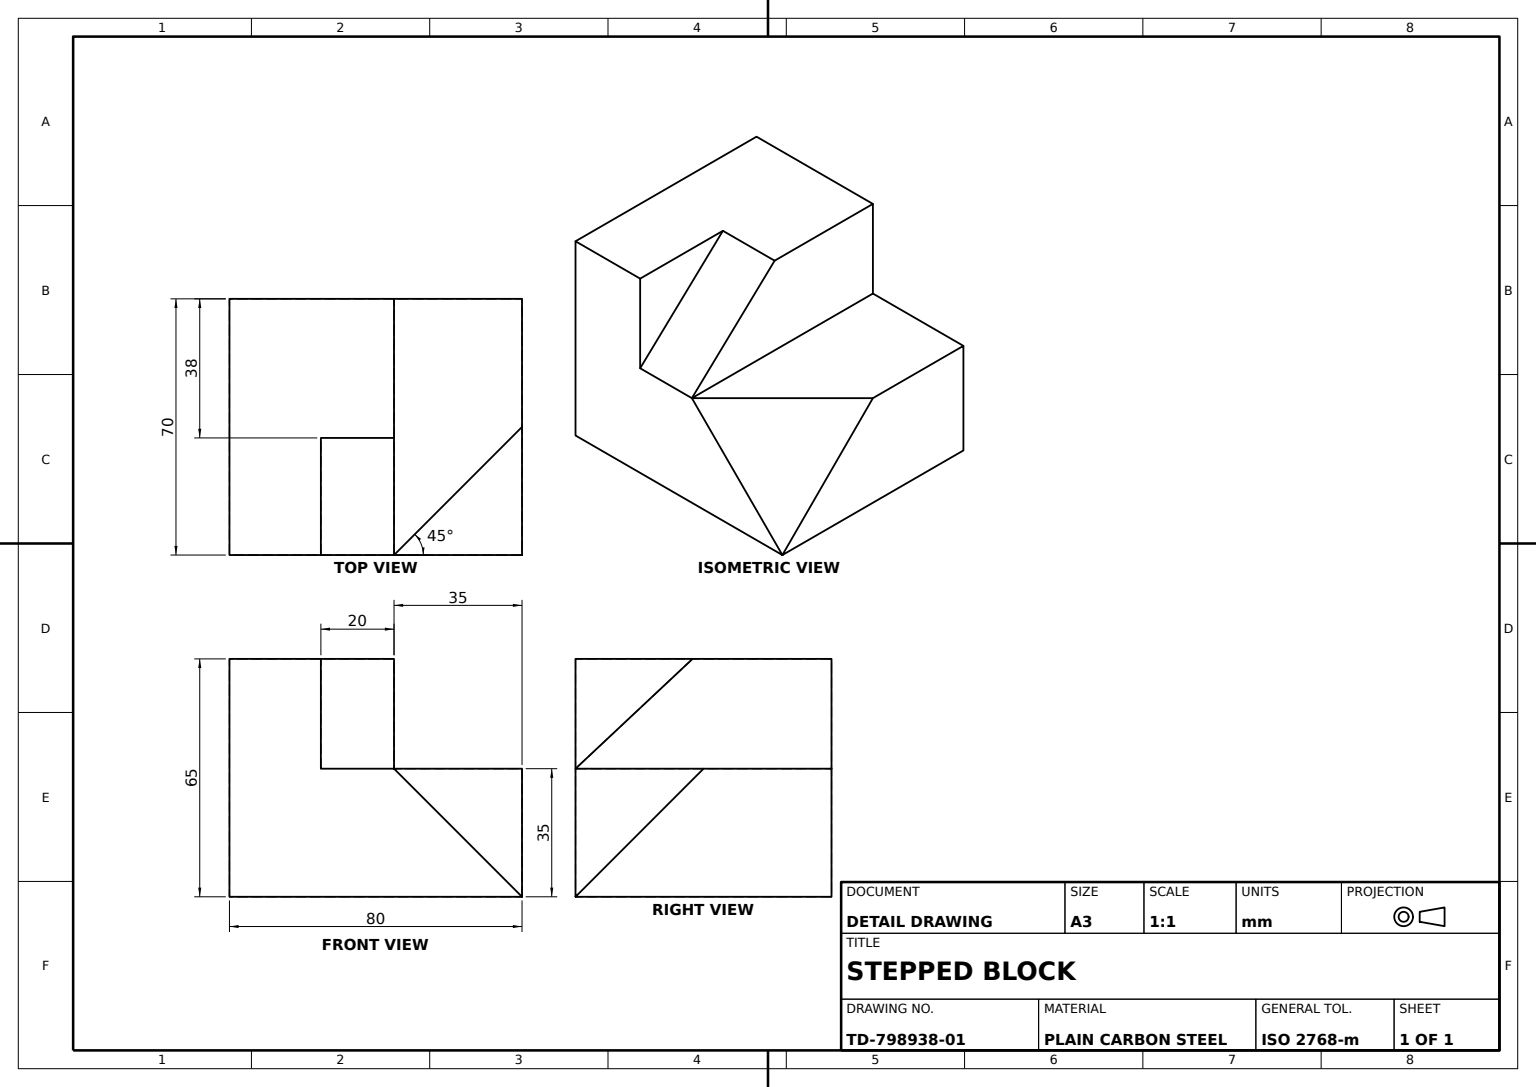
SolidWorks part; units mm, degrees
material "Plain Carbon Steel"
ref_plane "Front Plane" through (0, 0, 0) normal (0, 0, 1) x (1, 0, 0)
ref_plane "Top Plane" through (0, 0, 0) normal (0, 1, 0) x (1, 0, 0)
ref_plane "Right Plane" through (0, 0, 0) normal (1, 0, 0) x (0, 0, -1)
sketch "Block Profile Sketch 70x65" plane through (0, 0, 0) normal (0, 0, 1) x (1, 0, 0)
  line L0 (0, 0) -> (70, 0)
  line L1 (70, 0) -> (70, 65)
  line L2 (70, 65) -> (0, 65)
  line L3 (0, 65) -> (0, 0)
  dimension "D1" = 65
  dimension "D2" = 70
extrude "Base Block 70x65x80" add sketch "Block Profile Sketch 70x65" along normal mid plane 80
sketch "Upper Step Sketch" plane through (0, 0, 40) normal (0, 0, 1) x (1, 0, 0)
  line L0 (0, 35) -> (70, 35)
  line L1 (0, 65) -> (0, 0) construction
  line L2 (70, 0) -> (70, 65) construction
  line L3 (70, 35) -> (70, 65)
  line L4 (70, 65) -> (0, 65)
  line L5 (0, 65) -> (0, 35)
  line L6 (0, 0) -> (70, 0) construction
  dimension "D1" = 35
extrude "Upper Step Cut 35" cut sketch "Upper Step Sketch" against normal blind 35
sketch "Lower Step Sketch" plane through (0, 0, 5) normal (0, 0, 1) x (1, 0, 0)
  line L0 (0, 35) -> (32, 65)
  line L1 (70, 65) -> (0, 65) construction
  line L2 (70, 35) -> (70, 65) construction
  line L6 (0, 65) -> (0, 35) construction
  line L7 (32, 65) -> (0, 65)
  line L8 (0, 65) -> (0, 35)
  dimension "D1" = 38
extrude "Lower Step Cut 20" cut sketch "Lower Step Sketch" against normal blind 20
sketch3d "Corner Cut Reference 3D Sketch"
  line L0 (0, 0, 40) -> (35, 35, 40) construction
  line L1 (0, 35, 40) -> (70, 35, 40) construction
  line L2 (35, 35, 40) -> (0, 35, 5) construction
  line L3 (0, 35, 5) -> (0, 0, 40) construction
  line L4 (70, 35, 5) -> (70, 35, 40) construction
  dimension "D1" = 35
ref_plane "Corner Cut Plane" through (-13.3333, 13.3333, 13.3333) normal (0.5774, -0.5774, -0.5774) x (-0.8165, -0.4082, -0.4082)
sketch "Corner Cut Sketch" plane through (-13.3333, 13.3333, 13.3333) normal (0.5774, -0.5774, -0.5774) x (-0.8165, -0.4082, -0.4082)
  line L0 (-16.3299, 21.2132) -> (-16.3299, -28.2843) construction
  line L1 (-16.3299, -28.2843) -> (-59.196, -3.5355) construction
  line L2 (-59.196, -3.5355) -> (-16.3299, 21.2132) construction
  line L3 (-16.3299, 21.2132) -> (-16.3299, -28.2843)
  line L4 (-16.3299, -28.2843) -> (-59.196, -3.5355)
  line L5 (-59.196, -3.5355) -> (-16.3299, 21.2132)
extrude "Angled Corner Cut" cut sketch "Corner Cut Sketch" against normal blind 56
